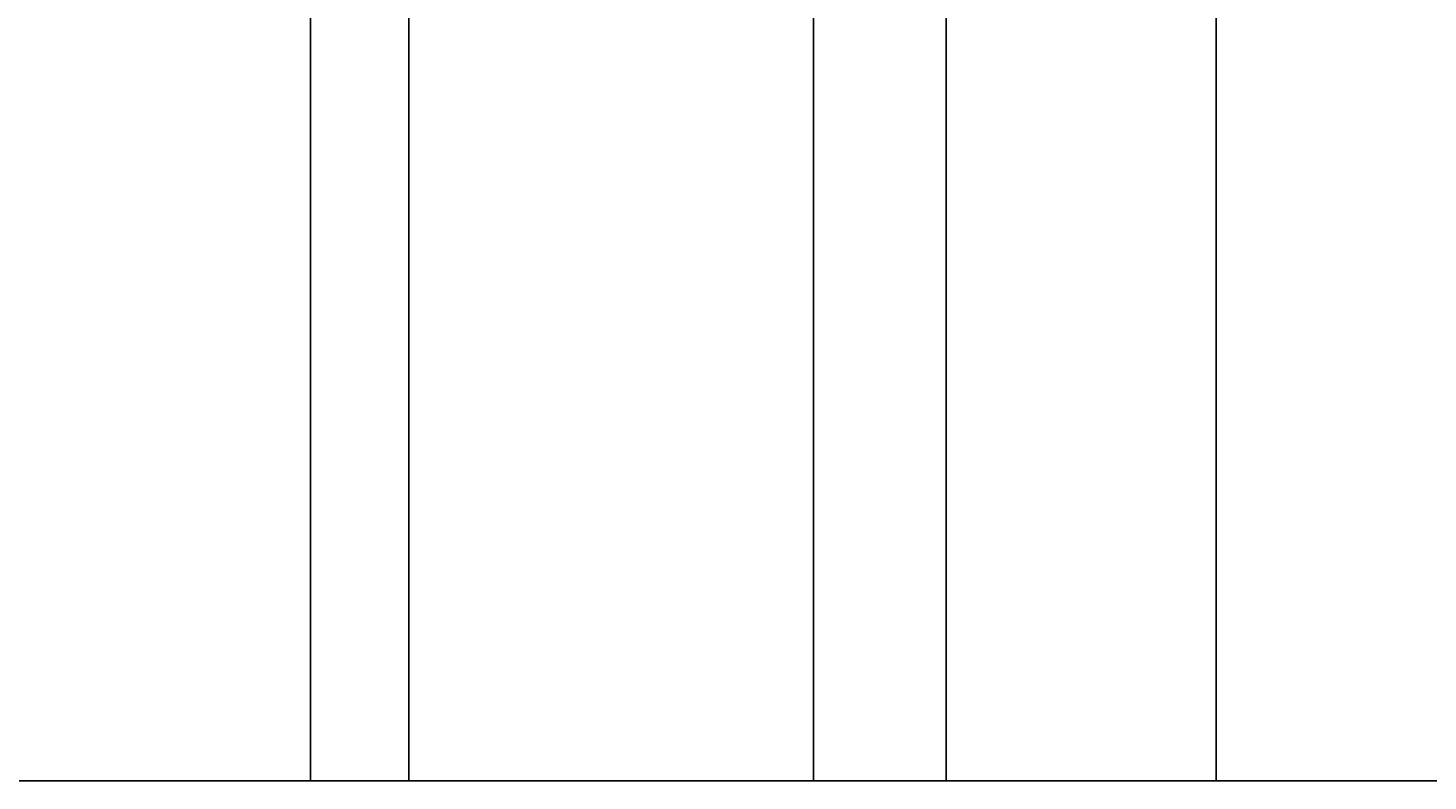
# Model space of a CAD drawing. Units: inches. Extents: x 35362 to 73946, y 43607 to 67532.
# Tile 49 of 134: x 49302 to 52380, y 43607 to 45263. Entities that reach past the tile are written whole.
import ezdxf

# ---------------------------------------------------------------- set-up
doc = ezdxf.new("R2010")
doc.units = ezdxf.units.IN
doc.header["$MEASUREMENT"] = 0
doc.layers.add('A-ANNO-DIMS', color=2, linetype='Continuous', lineweight=18)
doc.styles.get("Standard").update_dxf_attribs({"font": 'arial.ttf'})
doc.dimstyles.get("Standard").update_dxf_attribs({"dimtxt": 0.18, "dimasz": 0.18, "dimexe": 0.18, "dimexo": 0.0625, "dimgap": 0.09, "dimtad": 0, "dimtih": 1, "dimtoh": 1, "dimdec": 4, "dimzin": 0, "dimdsep": 46, "dimtxsty": 'Standard', "dimcen": 0.09, "dimadec": 0, "dimazin": 0, "dimtfac": 1, "dimtdec": 4, "dimtofl": 0, "dimtmove": 0, "dimatfit": 3, "dimfxl": 1, "dimtolj": 1, "dimtzin": 0, "dimarcsym": 0})

# ---------------------------------------------------------------- blocks, each defined once
blk = doc.blocks.new('*D5')
at = {"layer": 'A-ANNO-DIMS', "color": 0, "lineweight": -2, "transparency": 16777216}
for p, q in [((37121.9, 46919.3), (37121.9, 43606.7)), ((69871.5, 45449.8), (69871.5, 43606.7)), ((37122.1, 43606.9), (53496.3, 43606.9)), ((69871.3, 43606.9), (53497.2, 43606.9))]:
    blk.add_line(p, q, dxfattribs=at)
at = {"layer": 'A-ANNO-DIMS', "color": 0, "transparency": 16777216}
for points in [[(37122.1, 43606.9), (37122.1, 43606.8), (37121.9, 43606.9)], [(69871.3, 43606.9), (69871.3, 43606.8), (69871.5, 43606.9)]]:
    blk.add_solid(points, dxfattribs=at)
at = {"layer": 'Defpoints', "color": 0, "transparency": 16777216}
for p in [(37121.9, 46919.4), (69871.5, 45449.9), (69871.5, 43606.9)]:
    blk.add_point(p, dxfattribs=at)
at = {"layer": 'A-ANNO-DIMS', "color": 0, "transparency": 16777216, "insert": (53496.7, 43606.9), "char_height": 0.18, "attachment_point": 5}
blk.add_mtext('\\A1;32750', dxfattribs=at)
blk = doc.blocks.new('*D11')
at = {"layer": 'A-ANNO-DIMS', "color": 0, "lineweight": -2, "transparency": 16777216}
for p, q in [((47978.7, 56028.8), (47978.7, 43606.7)), ((53109.8, 56028.8), (53109.8, 43606.7)), ((47978.8, 43606.9), (50543.9, 43606.9)), ((53109.6, 43606.9), (50544.6, 43606.9))]:
    blk.add_line(p, q, dxfattribs=at)
at = {"layer": 'A-ANNO-DIMS', "color": 0, "transparency": 16777216}
for points in [[(47978.8, 43606.9), (47978.8, 43606.8), (47978.7, 43606.9)], [(53109.6, 43606.9), (53109.6, 43606.8), (53109.8, 43606.9)]]:
    blk.add_solid(points, dxfattribs=at)
at = {"layer": 'Defpoints', "color": 0, "transparency": 16777216}
for p in [(47978.7, 56028.8), (53109.8, 56028.8), (53109.8, 43606.9)]:
    blk.add_point(p, dxfattribs=at)
at = {"layer": 'A-ANNO-DIMS', "color": 0, "transparency": 16777216, "insert": (50544.2, 43606.9), "char_height": 0.18, "attachment_point": 5}
blk.add_mtext('\\A1;5131', dxfattribs=at)
blk = doc.blocks.new('*D13')
at = {"layer": 'A-ANNO-DIMS', "color": 0, "lineweight": -2, "transparency": 16777216}
for p, q in [((48373.5, 51694), (48373.5, 43606.7)), ((51029, 51694), (51029, 43606.7)), ((48373.7, 43606.9), (49700.8, 43606.9)), ((51028.9, 43606.9), (49701.7, 43606.9))]:
    blk.add_line(p, q, dxfattribs=at)
at = {"layer": 'A-ANNO-DIMS', "color": 0, "transparency": 16777216}
for points in [[(48373.7, 43606.9), (48373.7, 43606.8), (48373.5, 43606.9)], [(51028.9, 43606.9), (51028.9, 43606.8), (51029, 43606.9)]]:
    blk.add_solid(points, dxfattribs=at)
at = {"layer": 'Defpoints', "color": 0, "transparency": 16777216}
for p in [(48373.5, 51694.1), (51029, 51694.1), (51029, 43606.9)]:
    blk.add_point(p, dxfattribs=at)
at = {"layer": 'A-ANNO-DIMS', "color": 0, "transparency": 16777216, "insert": (49701.3, 43606.9), "char_height": 0.18, "attachment_point": 5}
blk.add_mtext('\\A1;2655.6', dxfattribs=at)
blk = doc.blocks.new('*D17')
at = {"layer": 'A-ANNO-DIMS', "color": 0, "lineweight": -2, "transparency": 16777216}
for p, q in [((49923.3, 61293.2), (49923.3, 43606.7)), ((51913.9, 61293.2), (51913.9, 43606.7)), ((49923.5, 43606.9), (50918.2, 43606.9)), ((51913.8, 43606.9), (50919.1, 43606.9))]:
    blk.add_line(p, q, dxfattribs=at)
at = {"layer": 'A-ANNO-DIMS', "color": 0, "transparency": 16777216}
for points in [[(49923.5, 43606.9), (49923.5, 43606.8), (49923.3, 43606.9)], [(51913.8, 43606.9), (51913.8, 43606.8), (51913.9, 43606.9)]]:
    blk.add_solid(points, dxfattribs=at)
at = {"layer": 'Defpoints', "color": 0, "transparency": 16777216}
for p in [(49923.3, 61293.3), (51913.9, 61293.3), (51913.9, 43606.9)]:
    blk.add_point(p, dxfattribs=at)
at = {"layer": 'A-ANNO-DIMS', "color": 0, "transparency": 16777216, "insert": (50918.6, 43606.9), "char_height": 0.18, "attachment_point": 5}
blk.add_mtext('\\A1;1990.6', dxfattribs=at)
blk = doc.blocks.new('*D107')
at = {"layer": 'A-ANNO-DIMS', "color": 0, "lineweight": -2, "transparency": 16777216}
for p, q in [((50139.6, 59850), (50139.6, 43606.7)), ((51320.8, 59850), (51320.8, 43606.7)), ((50139.7, 43606.9), (50729.7, 43606.9)), ((51320.6, 43606.9), (50730.6, 43606.9))]:
    blk.add_line(p, q, dxfattribs=at)
at = {"layer": 'A-ANNO-DIMS', "color": 0, "transparency": 16777216}
for points in [[(50139.7, 43606.9), (50139.7, 43606.8), (50139.6, 43606.9)], [(51320.6, 43606.9), (51320.6, 43606.8), (51320.8, 43606.9)]]:
    blk.add_solid(points, dxfattribs=at)
at = {"layer": 'Defpoints', "color": 0, "transparency": 16777216}
for p in [(50139.6, 59850.1), (51320.8, 59850.1), (51320.8, 43606.9)]:
    blk.add_point(p, dxfattribs=at)
at = {"layer": 'A-ANNO-DIMS', "color": 0, "transparency": 16777216, "insert": (50730.2, 43606.9), "char_height": 0.18, "attachment_point": 5}
blk.add_mtext('\\A1;1181.3', dxfattribs=at)

msp = doc.modelspace()

# ---------------------------------------------------------------- dimensions: what is measured, and where the dimension line sits
at = {"layer": 'A-ANNO-DIMS'}
for base, p1, p2, override, picture, middle in [((51913.931, 43606.859), (49923.307, 61293.286), (51913.931, 61293.286), {"dimdec": 1, "dimlfac": 1, "dimrnd": 0, "dimzin": 0, "dimdsep": 46, "dimlunit": 2}, '*D17', (50918.619, 43606.859)), ((51320.8133, 43606.859), (50139.5627, 59850.0769), (51320.8133, 59850.0769), {"dimdec": 1, "dimlfac": 1, "dimrnd": 0, "dimzin": 0, "dimdsep": 46, "dimlunit": 2}, '*D107', (50730.188, 43606.859)), ((53109.76, 43606.859), (47978.665, 56028.836), (53109.76, 56028.836), {"dimdec": 0, "dimlfac": 1, "dimrnd": 0, "dimzin": 0, "dimdsep": 46, "dimlunit": 2}, '*D11', (50544.212, 43606.859)), ((51029.043, 43606.859), (48373.492, 51694.087), (51029.043, 51694.087), {"dimdec": 1, "dimlfac": 1, "dimrnd": 0, "dimzin": 0, "dimdsep": 46, "dimlunit": 2}, '*D13', (49701.267, 43606.859)), ((69871.496, 43606.859), (37121.949, 46919.381), (69871.496, 45449.894), {"dimdec": 0, "dimlfac": 1, "dimrnd": 0, "dimzin": 0, "dimdsep": 46, "dimlunit": 2}, '*D5', (53496.723, 43606.859))]:
    dim = msp.add_linear_dim(base=base, p1=p1, p2=p2, dimstyle='Standard', override=override, dxfattribs=at)
    dim.commit()
    dim.dimension.update_dxf_attribs({"geometry": picture, "text_midpoint": middle})

doc.saveas('drawing.dxf')
